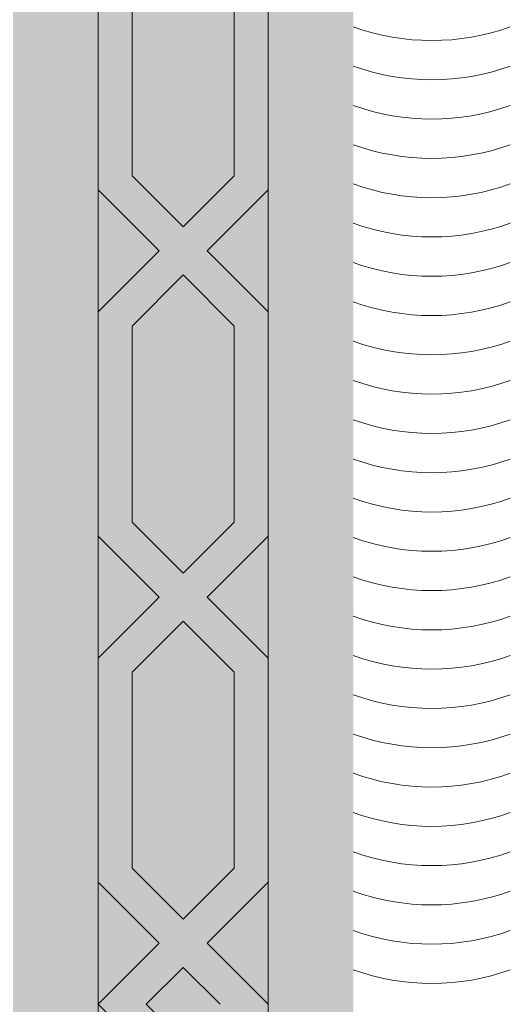
# Model space of a CAD drawing. Units: inches. Extents: x 844 to 2234, y 346 to 1084.
# Tile 61 of 93: x 1873.853 to 1877.533, y 701.365 to 708.747. Entities that reach past the tile are written whole.
import ezdxf

# ---------------------------------------------------------------- set-up
doc = ezdxf.new("R2010")
doc.units = ezdxf.units.IN
doc.header["$MEASUREMENT"] = 0
doc.layers.add('furniture', color=8, linetype='Continuous', lineweight=18)
doc.layers.add('RA-AP-01$0$INT', color=35, linetype='Continuous', lineweight=5)
doc.layers.add('RA-AP-01$0$FURN', color=3, linetype='Continuous')

# ---------------------------------------------------------------- blocks, each defined once
blk = doc.blocks.new('A$C18D01794')
at = {"layer": 'RA-AP-01$0$INT'}
h = blk.add_hatch(color=256, dxfattribs=at)
h.paths.add_polyline_path([(4.35521, -6.15671), (4.35521, -8.05671), (5.45521, -8.05671), (5.45521, -6.15671)])
h.paths.add_polyline_path([(4.40521, -8.00671), (4.40521, -6.20671), (5.40521, -6.20671), (5.40521, -8.00671)], flags=16)
h = blk.add_hatch(color=256, dxfattribs=at)
h.paths.add_polyline_path([(4.46935, -7.07085), (4.50521, -7.035), (4.50521, -7.10671)])
h.paths.add_polyline_path([(4.45521, -7.085), (4.47692, -7.10671), (4.43349, -7.10671)])
h.paths.add_polyline_path([(4.40521, -7.035), (4.44106, -7.07085), (4.40521, -7.10671)])
h.paths.add_polyline_path([(4.42521, -6.91146), (4.45521, -6.88146), (4.48521, -6.91146), (4.48521, -7.02671), (4.45521, -7.05671), (4.42521, -7.02671)])
h.paths.add_polyline_path([(4.50521, -6.83146), (4.50521, -6.90318), (4.46935, -6.86732)])
h.paths.add_polyline_path([(4.42521, -6.70793), (4.45521, -6.67793), (4.48521, -6.70793), (4.48521, -6.82318), (4.45521, -6.85318), (4.42521, -6.82318)])
h.paths.add_polyline_path([(4.42521, -6.50439), (4.45521, -6.47439), (4.48521, -6.50439), (4.48521, -6.61964), (4.45521, -6.64964), (4.42521, -6.61964)])
h.paths.add_polyline_path([(4.46935, -6.66378), (4.50521, -6.62793), (4.50521, -6.69964)])
h.paths.add_polyline_path([(4.40521, -6.62793), (4.44106, -6.66378), (4.40521, -6.69964)])
h.paths.add_polyline_path([(4.40521, -6.42439), (4.44106, -6.46025), (4.40521, -6.49611)])
h.paths.add_polyline_path([(4.46935, -6.46025), (4.50521, -6.42439), (4.50521, -6.49611)])
h.paths.add_polyline_path([(4.42521, -6.30085), (4.45521, -6.27085), (4.48521, -6.30085), (4.48521, -6.41611), (4.45521, -6.44611), (4.42521, -6.41611)])
h.paths.add_polyline_path([(4.42521, -6.22671), (4.47106, -6.22671), (4.42521, -6.27257)])
h.paths.add_polyline_path([(4.49935, -6.22671), (4.63606, -6.22671), (4.66606, -6.25671), (4.63606, -6.28671), (4.49935, -6.28671), (4.46935, -6.25671)])
h.paths.add_polyline_path([(4.68021, -6.27085), (4.71606, -6.30671), (4.64435, -6.30671)])
h.paths.add_polyline_path([(4.64435, -6.20671), (4.71606, -6.20671), (4.68021, -6.24257)])
h.paths.add_polyline_path([(4.72435, -6.22671), (4.86106, -6.22671), (4.89106, -6.25671), (4.86106, -6.28671), (4.72435, -6.28671), (4.69435, -6.25671)])
h.paths.add_polyline_path([(4.90521, -6.27085), (4.94106, -6.30671), (4.86935, -6.30671)])
h.paths.add_polyline_path([(4.86935, -6.20671), (4.94106, -6.20671), (4.90521, -6.24257)])
h.paths.add_polyline_path([(4.94935, -6.22671), (5.08606, -6.22671), (5.11606, -6.25671), (5.08606, -6.28671), (4.94935, -6.28671), (4.91935, -6.25671)])
h.paths.add_polyline_path([(5.13021, -6.27085), (5.16606, -6.30671), (5.09435, -6.30671)])
h.paths.add_polyline_path([(5.09435, -6.20671), (5.16606, -6.20671), (5.13021, -6.24257)])
h.paths.add_polyline_path([(5.17435, -6.22671), (5.31106, -6.22671), (5.34106, -6.25671), (5.31106, -6.28671), (5.17435, -6.28671), (5.14435, -6.25671)])
h.paths.add_polyline_path([(5.32521, -6.30085), (5.35521, -6.27085), (5.38521, -6.30085), (5.38521, -6.41611), (5.35521, -6.44611), (5.32521, -6.41611)])
h.paths.add_polyline_path([(5.33935, -6.22671), (5.38521, -6.22671), (5.38521, -6.27257)])
h.paths.add_polyline_path([(5.32521, -6.50439), (5.35521, -6.47439), (5.38521, -6.50439), (5.38521, -6.61964), (5.35521, -6.64964), (5.32521, -6.61964)])
h.paths.add_polyline_path([(5.30521, -6.42439), (5.34106, -6.46025), (5.30521, -6.49611)])
h.paths.add_polyline_path([(5.36935, -6.46025), (5.40521, -6.42439), (5.40521, -6.49611)])
h.paths.add_polyline_path([(5.40521, -6.62793), (5.40521, -6.69964), (5.36935, -6.66378)])
h.paths.add_polyline_path([(5.30521, -6.62793), (5.34106, -6.66378), (5.30521, -6.69964)])
h.paths.add_polyline_path([(5.32521, -6.70793), (5.35521, -6.67793), (5.38521, -6.70793), (5.38521, -6.82318), (5.35521, -6.85318), (5.32521, -6.82318)])
h.paths.add_polyline_path([(5.30521, -6.83146), (5.34106, -6.86732), (5.30521, -6.90318)])
h.paths.add_polyline_path([(5.32521, -6.91146), (5.35521, -6.88146), (5.38521, -6.91146), (5.38521, -7.02671), (5.35521, -7.05671), (5.32521, -7.02671)])
h.paths.add_polyline_path([(5.40458, -6.83209, 0.001218), (5.40521, -6.83231), (5.40521, -6.90318), (5.36935, -6.86732)])
h.paths.add_polyline_path([(5.36935, -7.07085), (5.40521, -7.035), (5.40521, -7.10671)])
h.paths.add_polyline_path([(5.35521, -7.085), (5.37692, -7.10671), (5.33349, -7.10671)])
h.paths.add_polyline_path([(5.30521, -7.035), (5.34106, -7.07085), (5.30521, -7.10671)])
h = blk.add_hatch(color=256, dxfattribs=at)
h.paths.add_polyline_path([(4.50521, -6.62793), (4.46935, -6.66378), (4.50521, -6.69964), (4.50521, -6.83146), (4.46935, -6.86732), (4.50521, -6.90318), (4.50521, -7.035), (4.46935, -7.07085), (4.50521, -7.10671), (4.47692, -7.10671), (4.45521, -7.085), (4.43349, -7.10671), (4.40521, -7.10671), (4.44106, -7.07085), (4.40521, -7.035), (4.40521, -6.90318), (4.44106, -6.86732), (4.40521, -6.83146), (4.40521, -6.69964), (4.44106, -6.66378), (4.40521, -6.62793), (4.40521, -6.49611), (4.44106, -6.46025), (4.40521, -6.42439), (4.40521, -6.20671), (4.64435, -6.20671), (4.68021, -6.24257), (4.71606, -6.20671), (4.86935, -6.20671), (4.90521, -6.24257), (4.94106, -6.20671), (5.09435, -6.20671), (5.13021, -6.24257), (5.16606, -6.20671), (5.40521, -6.20671), (5.40521, -6.42439), (5.36935, -6.46025), (5.40521, -6.49611), (5.40521, -6.62793), (5.36935, -6.66378), (5.40521, -6.69964), (5.40521, -6.83146), (5.36935, -6.86732), (5.40521, -6.90318), (5.40521, -7.035), (5.36935, -7.07085), (5.40521, -7.10671), (5.37692, -7.10671), (5.35521, -7.085), (5.33349, -7.10671), (5.30521, -7.10671), (5.34106, -7.07085), (5.30521, -7.035), (5.30521, -6.90318), (5.34106, -6.86732), (5.30521, -6.83146), (5.30521, -6.69964), (5.34106, -6.66378), (5.30521, -6.62793), (5.30521, -6.49611), (5.34106, -6.46025), (5.30521, -6.42439), (5.30521, -6.30671), (5.16606, -6.30671), (5.13021, -6.27085), (5.09435, -6.30671), (4.94106, -6.30671), (4.90521, -6.27085), (4.86935, -6.30671), (4.71606, -6.30671), (4.68021, -6.27085), (4.64435, -6.30671), (4.50521, -6.30671), (4.50521, -6.42439), (4.46935, -6.46025), (4.50521, -6.49611)])
h.paths.add_polyline_path([(4.48521, -6.50439), (4.45521, -6.47439), (4.42521, -6.50439), (4.42521, -6.61964), (4.45521, -6.64964), (4.48521, -6.61964)], flags=16)
h.paths.add_polyline_path([(4.45521, -6.44611), (4.48521, -6.41611), (4.48521, -6.30085), (4.45521, -6.27085), (4.42521, -6.30085), (4.42521, -6.41611)], flags=16)
h.paths.add_polyline_path([(4.45521, -6.67793), (4.42521, -6.70793), (4.42521, -6.82318), (4.45521, -6.85318), (4.48521, -6.82318), (4.48521, -6.70793)], flags=16)
h.paths.add_polyline_path([(4.49935, -6.28671), (4.63606, -6.28671), (4.66606, -6.25671), (4.63606, -6.22671), (4.49935, -6.22671), (4.46935, -6.25671)], flags=16)
h.paths.add_polyline_path([(4.42521, -6.27257), (4.47106, -6.22671), (4.42521, -6.22671)], flags=16)
h.paths.add_polyline_path([(4.45521, -6.88146), (4.42521, -6.91146), (4.42521, -7.02671), (4.45521, -7.05671), (4.48521, -7.02671), (4.48521, -6.91146)], flags=16)
h.paths.add_polyline_path([(4.72435, -6.28671), (4.86106, -6.28671), (4.89106, -6.25671), (4.86106, -6.22671), (4.72435, -6.22671), (4.69435, -6.25671)], flags=16)
h.paths.add_polyline_path([(4.91935, -6.25671), (4.94935, -6.28671), (5.08606, -6.28671), (5.11606, -6.25671), (5.08606, -6.22671), (4.94935, -6.22671)], flags=16)
h.paths.add_polyline_path([(5.14435, -6.25671), (5.17435, -6.28671), (5.31106, -6.28671), (5.34106, -6.25671), (5.31106, -6.22671), (5.17435, -6.22671)], flags=16)
h.paths.add_polyline_path([(5.32521, -6.61964), (5.35521, -6.64964), (5.38521, -6.61964), (5.38521, -6.50439), (5.35521, -6.47439), (5.32521, -6.50439)], flags=16)
h.paths.add_polyline_path([(5.32521, -6.41611), (5.35521, -6.44611), (5.38521, -6.41611), (5.38521, -6.30085), (5.35521, -6.27085), (5.32521, -6.30085)], flags=16)
h.paths.add_polyline_path([(5.32521, -6.70793), (5.32521, -6.82318), (5.35521, -6.85318), (5.38521, -6.82318), (5.38521, -6.70793), (5.35521, -6.67793)], flags=16)
h.paths.add_polyline_path([(5.32521, -6.91146), (5.32521, -7.02671), (5.35521, -7.05671), (5.38521, -7.02671), (5.38521, -6.91146), (5.35521, -6.88146)], flags=16)
h.paths.add_polyline_path([(5.33935, -6.22671), (5.38521, -6.27257), (5.38521, -6.22671)], flags=16)
for points in [[(4.50521, -6.30671), (5.30521, -6.30671), (5.30521, -7.10671), (5.25521, -7.10671), (5.25521, -6.35671), (4.55521, -6.35671), (4.55521, -7.10671), (4.50521, -7.10671)], [(4.50521, -7.90671), (5.30521, -7.90671), (5.30521, -7.10671), (5.25521, -7.10671), (5.25521, -7.85671), (4.55521, -7.85671), (4.55521, -7.10671), (4.50521, -7.10671)]]:
    blk.add_hatch(color=256, dxfattribs=at).paths.add_polyline_path(points)
h = blk.add_hatch(color=256, dxfattribs=at)
h.paths.add_polyline_path([(4.50521, -7.5855), (4.46935, -7.54964), (4.50521, -7.51378), (4.50521, -7.38196), (4.46935, -7.34611), (4.50521, -7.31025), (4.50521, -7.17843), (4.46935, -7.14257), (4.50521, -7.10671), (4.47692, -7.10671), (4.45521, -7.12843), (4.43349, -7.10671), (4.40521, -7.10671), (4.44106, -7.14257), (4.40521, -7.17843), (4.40521, -7.31025), (4.44106, -7.34611), (4.40521, -7.38196), (4.40521, -7.51378), (4.44106, -7.54964), (4.40521, -7.5855), (4.40521, -7.71732), (4.44106, -7.75318), (4.40521, -7.78903), (4.40521, -8.00671), (4.64435, -8.00671), (4.68021, -7.97085), (4.71606, -8.00671), (4.86935, -8.00671), (4.90521, -7.97085), (4.94106, -8.00671), (5.09435, -8.00671), (5.13021, -7.97085), (5.16606, -8.00671), (5.40521, -8.00671), (5.40521, -7.78903), (5.36935, -7.75318), (5.40521, -7.71732), (5.40521, -7.5855), (5.36935, -7.54964), (5.40521, -7.51378), (5.40521, -7.38196), (5.36935, -7.34611), (5.40521, -7.31025), (5.40521, -7.17843), (5.36935, -7.14257), (5.40521, -7.10671), (5.37692, -7.10671), (5.35521, -7.12843), (5.33349, -7.10671), (5.30521, -7.10671), (5.34106, -7.14257), (5.30521, -7.17843), (5.30521, -7.31025), (5.34106, -7.34611), (5.30521, -7.38196), (5.30521, -7.51378), (5.34106, -7.54964), (5.30521, -7.5855), (5.30521, -7.71732), (5.34106, -7.75318), (5.30521, -7.78903), (5.30521, -7.90671), (5.16606, -7.90671), (5.13021, -7.94257), (5.09435, -7.90671), (4.94106, -7.90671), (4.90521, -7.94257), (4.86935, -7.90671), (4.71606, -7.90671), (4.68021, -7.94257), (4.64435, -7.90671), (4.50521, -7.90671), (4.50521, -7.78903), (4.46935, -7.75318), (4.50521, -7.71732)])
h.paths.add_polyline_path([(4.48521, -7.70903), (4.45521, -7.73903), (4.42521, -7.70903), (4.42521, -7.59378), (4.45521, -7.56378), (4.48521, -7.59378)], flags=16)
h.paths.add_polyline_path([(4.45521, -7.76732), (4.48521, -7.79732), (4.48521, -7.91257), (4.45521, -7.94257), (4.42521, -7.91257), (4.42521, -7.79732)], flags=16)
h.paths.add_polyline_path([(4.45521, -7.5355), (4.42521, -7.5055), (4.42521, -7.39025), (4.45521, -7.36025), (4.48521, -7.39025), (4.48521, -7.5055)], flags=16)
h.paths.add_polyline_path([(4.49935, -7.92671), (4.63606, -7.92671), (4.66606, -7.95671), (4.63606, -7.98671), (4.49935, -7.98671), (4.46935, -7.95671)], flags=16)
h.paths.add_polyline_path([(4.42521, -7.94085), (4.47106, -7.98671), (4.42521, -7.98671)], flags=16)
h.paths.add_polyline_path([(4.45521, -7.33196), (4.42521, -7.30196), (4.42521, -7.18671), (4.45521, -7.15671), (4.48521, -7.18671), (4.48521, -7.30196)], flags=16)
h.paths.add_polyline_path([(4.72435, -7.92671), (4.86106, -7.92671), (4.89106, -7.95671), (4.86106, -7.98671), (4.72435, -7.98671), (4.69435, -7.95671)], flags=16)
h.paths.add_polyline_path([(4.91935, -7.95671), (4.94935, -7.92671), (5.08606, -7.92671), (5.11606, -7.95671), (5.08606, -7.98671), (4.94935, -7.98671)], flags=16)
h.paths.add_polyline_path([(5.14435, -7.95671), (5.17435, -7.92671), (5.31106, -7.92671), (5.34106, -7.95671), (5.31106, -7.98671), (5.17435, -7.98671)], flags=16)
h.paths.add_polyline_path([(5.32521, -7.59378), (5.35521, -7.56378), (5.38521, -7.59378), (5.38521, -7.70903), (5.35521, -7.73903), (5.32521, -7.70903)], flags=16)
h.paths.add_polyline_path([(5.32521, -7.79732), (5.35521, -7.76732), (5.38521, -7.79732), (5.38521, -7.91257), (5.35521, -7.94257), (5.32521, -7.91257)], flags=16)
h.paths.add_polyline_path([(5.32521, -7.5055), (5.32521, -7.39025), (5.35521, -7.36025), (5.38521, -7.39025), (5.38521, -7.5055), (5.35521, -7.5355)], flags=16)
h.paths.add_polyline_path([(5.32521, -7.30196), (5.32521, -7.18671), (5.35521, -7.15671), (5.38521, -7.18671), (5.38521, -7.30196), (5.35521, -7.33196)], flags=16)
h.paths.add_polyline_path([(5.33935, -7.98671), (5.38521, -7.94085), (5.38521, -7.98671)], flags=16)
h = blk.add_hatch(color=256, dxfattribs=at)
h.paths.add_polyline_path([(4.46935, -7.14257), (4.50521, -7.17843), (4.50521, -7.10671)])
h.paths.add_polyline_path([(4.45521, -7.12843), (4.47692, -7.10671), (4.43349, -7.10671)])
h.paths.add_polyline_path([(4.40521, -7.17843), (4.44106, -7.14257), (4.40521, -7.10671)])
h.paths.add_polyline_path([(4.42521, -7.30196), (4.45521, -7.33196), (4.48521, -7.30196), (4.48521, -7.18671), (4.45521, -7.15671), (4.42521, -7.18671)])
h.paths.add_polyline_path([(4.50521, -7.38196), (4.50521, -7.31025), (4.46935, -7.34611)])
h.paths.add_polyline_path([(4.42521, -7.5055), (4.45521, -7.5355), (4.48521, -7.5055), (4.48521, -7.39025), (4.45521, -7.36025), (4.42521, -7.39025)])
h.paths.add_polyline_path([(4.42521, -7.70903), (4.45521, -7.73903), (4.48521, -7.70903), (4.48521, -7.59378), (4.45521, -7.56378), (4.42521, -7.59378)])
h.paths.add_polyline_path([(4.46935, -7.54964), (4.50521, -7.5855), (4.50521, -7.51378)])
h.paths.add_polyline_path([(4.40521, -7.5855), (4.44106, -7.54964), (4.40521, -7.51378)])
h.paths.add_polyline_path([(4.40521, -7.78903), (4.44106, -7.75318), (4.40521, -7.71732)])
h.paths.add_polyline_path([(4.46935, -7.75318), (4.50521, -7.78903), (4.50521, -7.71732)])
h.paths.add_polyline_path([(4.42521, -7.91257), (4.45521, -7.94257), (4.48521, -7.91257), (4.48521, -7.79732), (4.45521, -7.76732), (4.42521, -7.79732)])
h.paths.add_polyline_path([(4.42521, -7.98671), (4.47106, -7.98671), (4.42521, -7.94085)])
h.paths.add_polyline_path([(4.49935, -7.98671), (4.63606, -7.98671), (4.66606, -7.95671), (4.63606, -7.92671), (4.49935, -7.92671), (4.46935, -7.95671)])
h.paths.add_polyline_path([(4.68021, -7.94257), (4.71606, -7.90671), (4.64435, -7.90671)])
h.paths.add_polyline_path([(4.64435, -8.00671), (4.71606, -8.00671), (4.68021, -7.97085)])
h.paths.add_polyline_path([(4.72435, -7.98671), (4.86106, -7.98671), (4.89106, -7.95671), (4.86106, -7.92671), (4.72435, -7.92671), (4.69435, -7.95671)])
h.paths.add_polyline_path([(4.90521, -7.94257), (4.94106, -7.90671), (4.86935, -7.90671)])
h.paths.add_polyline_path([(4.86935, -8.00671), (4.94106, -8.00671), (4.90521, -7.97085)])
h.paths.add_polyline_path([(4.94935, -7.98671), (5.08606, -7.98671), (5.11606, -7.95671), (5.08606, -7.92671), (4.94935, -7.92671), (4.91935, -7.95671)])
h.paths.add_polyline_path([(5.13021, -7.94257), (5.16606, -7.90671), (5.09435, -7.90671)])
h.paths.add_polyline_path([(5.09435, -8.00671), (5.16606, -8.00671), (5.13021, -7.97085)])
h.paths.add_polyline_path([(5.17435, -7.98671), (5.31106, -7.98671), (5.34106, -7.95671), (5.31106, -7.92671), (5.17435, -7.92671), (5.14435, -7.95671)])
h.paths.add_polyline_path([(5.32521, -7.91257), (5.35521, -7.94257), (5.38521, -7.91257), (5.38521, -7.79732), (5.35521, -7.76732), (5.32521, -7.79732)])
h.paths.add_polyline_path([(5.33935, -7.98671), (5.38521, -7.98671), (5.38521, -7.94085)])
h.paths.add_polyline_path([(5.32521, -7.70903), (5.35521, -7.73903), (5.38521, -7.70903), (5.38521, -7.59378), (5.35521, -7.56378), (5.32521, -7.59378)])
h.paths.add_polyline_path([(5.30521, -7.78903), (5.34106, -7.75318), (5.30521, -7.71732)])
h.paths.add_polyline_path([(5.36935, -7.75318), (5.40521, -7.78903), (5.40521, -7.71732)])
h.paths.add_polyline_path([(5.40521, -7.5855), (5.40521, -7.51378), (5.36935, -7.54964)])
h.paths.add_polyline_path([(5.30521, -7.5855), (5.34106, -7.54964), (5.30521, -7.51378)])
h.paths.add_polyline_path([(5.32521, -7.5055), (5.35521, -7.5355), (5.38521, -7.5055), (5.38521, -7.39025), (5.35521, -7.36025), (5.32521, -7.39025)])
h.paths.add_polyline_path([(5.30521, -7.38196), (5.34106, -7.34611), (5.30521, -7.31025)])
h.paths.add_polyline_path([(5.32521, -7.30196), (5.35521, -7.33196), (5.38521, -7.30196), (5.38521, -7.18671), (5.35521, -7.15671), (5.32521, -7.18671)])
h.paths.add_polyline_path([(5.40458, -7.38134, -0.001218), (5.40521, -7.38111), (5.40521, -7.31025), (5.36935, -7.34611)])
h.paths.add_polyline_path([(5.36935, -7.14257), (5.40521, -7.17843), (5.40521, -7.10671)])
h.paths.add_polyline_path([(5.35521, -7.12843), (5.37692, -7.10671), (5.33349, -7.10671)])
h.paths.add_polyline_path([(5.30521, -7.17843), (5.34106, -7.14257), (5.30521, -7.10671)])
for p, q in [((5.34106, -7.07085), (5.30521, -7.10671)), ((5.35521, -7.085), (5.33349, -7.10671)), ((5.34106, -7.14257), (5.30521, -7.10671)), ((5.35521, -7.12843), (5.33349, -7.10671)), ((5.35521, -7.12843), (5.37692, -7.10671)), ((5.36935, -7.14257), (5.40521, -7.10671)), ((5.30521, -7.17843), (5.34106, -7.14257)), ((5.40521, -7.17843), (5.36935, -7.14257)), ((5.32521, -7.18671), (5.35521, -7.15671)), ((5.38521, -7.18671), (5.35521, -7.15671)), ((5.32521, -7.30196), (5.32521, -7.18671)), ((5.38521, -7.30196), (5.38521, -7.18671)), ((5.32521, -7.30196), (5.35521, -7.33196)), ((5.38521, -7.30196), (5.35521, -7.33196)), ((5.30521, -7.31025), (5.34106, -7.34611)), ((5.40521, -7.31025), (5.36935, -7.34611)), ((5.30521, -7.38196), (5.34106, -7.34611)), ((5.40521, -7.38196), (5.36935, -7.34611)), ((5.32521, -7.39025), (5.35521, -7.36025)), ((5.38521, -7.39025), (5.35521, -7.36025)), ((5.32521, -7.39025), (5.32521, -7.5055)), ((5.38521, -7.39025), (5.38521, -7.5055)), ((5.32521, -7.5055), (5.35521, -7.5355)), ((5.38521, -7.5055), (5.35521, -7.5355)), ((5.30521, -7.51378), (5.34106, -7.54964)), ((5.40521, -7.51378), (5.36935, -7.54964)), ((5.30521, -7.5855), (5.34106, -7.54964)), ((5.40521, -7.5855), (5.36935, -7.54964)), ((5.32521, -7.59378), (5.35521, -7.56378)), ((5.38521, -7.59378), (5.35521, -7.56378)), ((5.32521, -7.59378), (5.32521, -7.70903)), ((5.38521, -7.59378), (5.38521, -7.70903))]:
    blk.add_line(p, q, dxfattribs=at)
for points in [[(5.40521, -7.10671), (5.40521, -6.20671)], [(5.30521, -7.10671), (5.30521, -6.30671), (4.50521, -6.30671), (4.50521, -7.10671)], [(5.30521, -7.10671), (5.30521, -7.90671), (4.50521, -7.90671), (4.50521, -7.10671)], [(5.40521, -7.10671), (5.40521, -8.00671)]]:
    blk.add_lwpolyline(points, dxfattribs=at)
for centre in [(5.50141, -7.25536), (5.50141, -7.27846), (5.50141, -7.30156), (5.50141, -7.32466), (5.50141, -7.34776), (5.50141, -7.37086), (5.50141, -7.39396), (5.50141, -7.41706), (5.50141, -7.44016), (5.50141, -7.46326), (5.50141, -7.48636), (5.50141, -7.50946), (5.50141, -7.53256), (5.50141, -7.55566), (5.50141, -7.57876), (5.50141, -7.60186), (5.50141, -7.62496), (5.50141, -7.64806), (5.50141, -7.67116), (5.50141, -7.67116), (5.50141, -7.69426), (5.50141, -7.71736), (5.50141, -7.74046), (5.50141, -7.76356), (5.50141, -7.78666), (5.50141, -7.80976)]:
    blk.add_arc(centre, 0.13641, 70.20384, 109.79616, dxfattribs=at)
blk = doc.blocks.new('A$C5D2F253E')
at = {"layer": 'RA-AP-01$0$FURN', "xscale": -0.7999999999883585, "yscale": 0.7999999999883585, "zscale": 0.8, "rotation": 90}
blk.add_blockref('A$C18D01794', (-5.68776, 4.75792), dxfattribs=at)

msp = doc.modelspace()

# ---------------------------------------------------------------- block references
at = {"layer": 'furniture', "xscale": 15.94108302203742, "yscale": 15.94108302203742, "zscale": 15.94108302203742, "rotation": 90}
msp.add_blockref('A$C5D2F253E', (1882.6311, 701.4029), dxfattribs=at)

doc.saveas('drawing.dxf')
